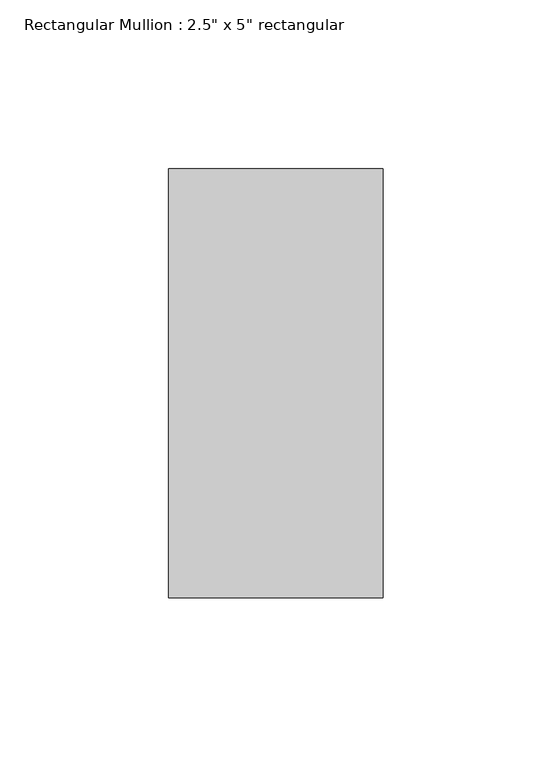
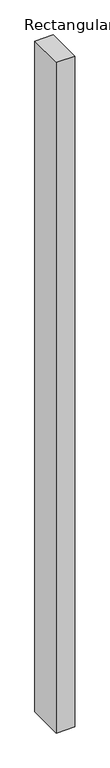
"""IFC4 building model written with IfcOpenShell, lengths in millimetres: member geometry."""

from ifc_helpers import new_model, si_unit, frame, origin, place, context, project, spatial, polyline, outline, extrude, source, transform, mapped, element, save


def member_ee409385(model_context):
    return source(origin(), model_context, "Body", "SweptSolid", [
        extrude(outline(polyline([(0.0, 63.5), (0.0, -63.5), (-63.5, -63.5), (-63.5, 63.5), (0.0, 63.5)])), frame((0.0, 0.0, -2438.4), z_axis=(0.0, 0.0, 1.0), x_axis=(1.0, 0.0, 0.0)), (0.0, 0.0, 1.0), 2438.4),
    ])


if __name__ == "__main__":
    model = new_model("IFC4")
    model_context = context("Model", 3, world=origin())
    ifc_project = project(units=[si_unit("LENGTHUNIT", "METRE", prefix="MILLI")], contexts=[model_context])
    site = spatial("IfcSite", under=ifc_project)
    building = spatial("IfcBuilding", under=site)
    placement = place(None, origin())
    member_shape = member_ee409385(model_context)
    element("IfcMember", 1, ObjectType="Rectangular Mullion : 2.5\" x 5\" rectangular", at=placement, inside=building, context=model_context, shape_type="MappedRepresentation", body=[
        mapped(member_shape, transform((0.0, 0.0, 0.0), x_axis=(1.0, 0.0, 0.0), y_axis=(0.0, 1.0, 0.0), z_axis=(0.0, 0.0, 1.0))),
    ])
    save(model, "model.ifc")

# Revit data of these elements
# Type "Rectangular Mullion : 2.5\" x 5\" rectangular"
#   built-in parameter 1007304 = 0.416667 (stored number, unit not read)
#   built-in parameter 1007301 = 0.104167 (stored number, unit not read)
#   built-in parameter 1007300 = 0.104167 (stored number, unit not read)
# Element 1 (IfcMember, "Rectangular Mullion : 2.5\" x 5\" rectangular")
#   Materials on its faces: "WINDOW FRAMING"
# Materials
#   "WINDOW FRAMING": class "Generic", colour RGB 120 120 120, transparency 0, Cost = 0
